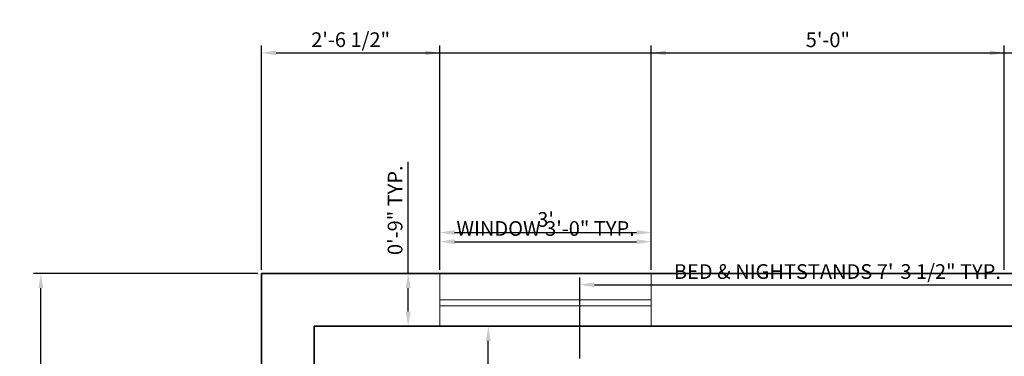
# Model space of a CAD drawing. Units: inches. Extents: x 2025 to 2528, y 1525 to 2336.
# Tile 13 of 18: x 2025 to 2192, y 2278 to 2336. Entities that reach past the tile are written whole.
import ezdxf

# ---------------------------------------------------------------- set-up
doc = ezdxf.new("R2010")
doc.units = ezdxf.units.IN
for name, color, linetype, lineweight in [('A-ANNO-DIMS', 2, 'Continuous', 18), ('A-GLAZ', 4, 'Continuous', 18), ('A-WALL', 7, 'Continuous', 35)]:
    doc.layers.add(name, color=color, linetype=linetype, lineweight=lineweight)
doc.styles.get("Standard").update_dxf_attribs({"font": 'arial.ttf'})
doc.dimstyles.new('Copy of ISO-25', dxfattribs={"dimtxt": 2.5, "dimasz": 2.5, "dimexe": 1.25, "dimexo": 0.625, "dimtad": 1, "dimdec": 1, "dimlunit": 4, "dimtxsty": 'Standard', "dimcen": 2.5, "dimadec": 0, "dimazin": 0, "dimtfac": 1, "dimtdec": 1, "dimtmove": 0, "dimatfit": 3, "dimfxl": 1, "dimarcsym": 0})

# ---------------------------------------------------------------- blocks, each defined once
blk = doc.blocks.new('*D6')
at = {"layer": 'A-ANNO-DIMS', "color": 0, "lineweight": -2, "transparency": 16777216}
for p, q in [((2075.01, 2282.79), (2075.01, 2237.93)), ((2255.01, 2282.79), (2255.01, 2237.93)), ((2077.51, 2239.18), (2252.51, 2239.18))]:
    blk.add_line(p, q, dxfattribs=at)
at = {"layer": 'A-ANNO-DIMS', "color": 0, "transparency": 16777216}
for points in [[(2077.51, 2239.59), (2077.51, 2238.76), (2075.01, 2239.18)], [(2252.51, 2239.59), (2252.51, 2238.76), (2255.01, 2239.18)]]:
    blk.add_solid(points, dxfattribs=at)
at = {"layer": 'Defpoints', "color": 0, "transparency": 16777216}
for p in [(2075.01, 2283.41), (2255.01, 2283.41), (2255.01, 2239.18)]:
    blk.add_point(p, dxfattribs=at)
at = {"layer": 'A-ANNO-DIMS', "color": 0, "transparency": 16777216, "insert": (2165.01, 2241.08), "char_height": 2.5, "attachment_point": 5}
blk.add_mtext("15'", dxfattribs=at)
blk = doc.blocks.new('*D7')
at = {"layer": 'A-ANNO-DIMS', "color": 0, "lineweight": -2, "transparency": 16777216}
for p, q in [((2075.64, 2283.41), (2105.88, 2283.41)), ((2104.63, 2117.91), (2104.63, 2280.91)), ((2075.64, 2115.41), (2105.88, 2115.41))]:
    blk.add_line(p, q, dxfattribs=at)
at = {"layer": 'A-ANNO-DIMS', "color": 0, "transparency": 16777216}
for points in [[(2104.22, 2280.91), (2105.05, 2280.91), (2104.63, 2283.41)], [(2104.22, 2117.91), (2105.05, 2117.91), (2104.63, 2115.41)]]:
    blk.add_solid(points, dxfattribs=at)
at = {"layer": 'Defpoints', "color": 0, "transparency": 16777216}
for p in [(2075.01, 2283.41), (2104.63, 2283.41), (2075.01, 2115.41)]:
    blk.add_point(p, dxfattribs=at)
at = {"layer": 'A-ANNO-DIMS', "color": 0, "transparency": 16777216, "insert": (2102.75, 2199.41), "char_height": 2.5, "attachment_point": 5, "rotation": 90}
blk.add_mtext("14'", dxfattribs=at)
blk = doc.blocks.new('*D22')
at = {"layer": 'A-ANNO-DIMS', "color": 0, "lineweight": -2, "transparency": 16777216}
for p, q in [((2096.39, 2293.04), (2096.39, 2300.62)), ((2132.39, 2293.04), (2132.39, 2300.62)), ((2098.89, 2299.37), (2129.89, 2299.37))]:
    blk.add_line(p, q, dxfattribs=at)
at = {"layer": 'A-ANNO-DIMS', "color": 0, "transparency": 16777216}
for points in [[(2098.89, 2299.78), (2098.89, 2298.95), (2096.39, 2299.37)], [(2129.89, 2299.78), (2129.89, 2298.95), (2132.39, 2299.37)]]:
    blk.add_solid(points, dxfattribs=at)
at = {"layer": 'Defpoints', "color": 0, "transparency": 16777216}
for p in [(2132.39, 2299.37), (2096.39, 2292.41), (2132.39, 2292.41)]:
    blk.add_point(p, dxfattribs=at)
at = {"layer": 'A-ANNO-DIMS', "color": 0, "transparency": 16777216, "insert": (2114.39, 2301.27), "char_height": 2.5, "attachment_point": 5}
blk.add_mtext("3'", dxfattribs=at)
blk = doc.blocks.new('WIN-36-EXT')
for p, q in [((0, 0), (0, 9)), ((0, 9), (36, 9)), ((36, 9), (36, 0)), ((0, 4.5), (36, 4.5)), ((0, 3.5), (36, 3.5))]:
    blk.add_line(p, q)
blk = doc.blocks.new('*D54')
at = {"layer": 'A-ANNO-DIMS', "color": 0, "lineweight": -2, "transparency": 16777216}
for p, q in [((2096.39, 2293.04), (2096.39, 2299.06)), ((2132.39, 2293.04), (2132.39, 2299.06)), ((2098.89, 2297.81), (2129.89, 2297.81))]:
    blk.add_line(p, q, dxfattribs=at)
at = {"layer": 'A-ANNO-DIMS', "color": 0, "transparency": 16777216}
for points in [[(2098.89, 2298.23), (2098.89, 2297.4), (2096.39, 2297.81)], [(2129.89, 2298.23), (2129.89, 2297.4), (2132.39, 2297.81)]]:
    blk.add_solid(points, dxfattribs=at)
at = {"layer": 'Defpoints', "color": 0, "transparency": 16777216}
for p in [(2132.39, 2297.81), (2096.39, 2292.41), (2132.39, 2292.41)]:
    blk.add_point(p, dxfattribs=at)
at = {"layer": 'A-ANNO-DIMS', "color": 0, "transparency": 16777216, "insert": (2114.39, 2299.73), "char_height": 2.5, "attachment_point": 5}
blk.add_mtext('WINDOW 3\'-0" TYP.', dxfattribs=at)
blk = doc.blocks.new('*D55')
at = {"layer": 'A-ANNO-DIMS', "color": 0, "lineweight": -2, "transparency": 16777216}
for p, q in [((2090.99, 2292.41), (2090.99, 2311.4)), ((2095.76, 2292.41), (2089.74, 2292.41)), ((2090.99, 2285.91), (2090.99, 2289.91)), ((2095.76, 2283.41), (2089.74, 2283.41))]:
    blk.add_line(p, q, dxfattribs=at)
at = {"layer": 'A-ANNO-DIMS', "color": 0, "transparency": 16777216}
for points in [[(2090.57, 2289.91), (2091.41, 2289.91), (2090.99, 2292.41)], [(2090.57, 2285.91), (2091.41, 2285.91), (2090.99, 2283.41)]]:
    blk.add_solid(points, dxfattribs=at)
at = {"layer": 'Defpoints', "color": 0, "transparency": 16777216}
for p in [(2090.99, 2292.41), (2096.39, 2292.41), (2096.39, 2283.41)]:
    blk.add_point(p, dxfattribs=at)
at = {"layer": 'A-ANNO-DIMS', "color": 0, "transparency": 16777216, "insert": (2089.09, 2303.16), "char_height": 2.5, "attachment_point": 5, "rotation": 90}
blk.add_mtext('0\'-9" TYP.', dxfattribs=at)
blk = doc.blocks.new('*D56')
at = {"layer": 'A-ANNO-DIMS', "color": 0, "lineweight": -2, "transparency": 16777216}
for p, q in [((2120.21, 2277.94), (2120.21, 2291.73)), ((2207.93, 2277.94), (2207.93, 2291.73)), ((2122.71, 2290.48), (2205.43, 2290.48))]:
    blk.add_line(p, q, dxfattribs=at)
at = {"layer": 'A-ANNO-DIMS', "color": 0, "transparency": 16777216}
for points in [[(2122.71, 2290.89), (2122.71, 2290.06), (2120.21, 2290.48)], [(2205.43, 2290.89), (2205.43, 2290.06), (2207.93, 2290.48)]]:
    blk.add_solid(points, dxfattribs=at)
at = {"layer": 'Defpoints', "color": 0, "transparency": 16777216}
for p in [(2207.93, 2290.48), (2120.21, 2277.32), (2207.93, 2277.32)]:
    blk.add_point(p, dxfattribs=at)
at = {"layer": 'A-ANNO-DIMS', "color": 0, "transparency": 16777216, "insert": (2164.07, 2292.4), "char_height": 2.5, "attachment_point": 5}
blk.add_mtext('BED & NIGHTSTANDS 7\'-3 1/2" TYP.', dxfattribs=at)
blk = doc.blocks.new('*D60')
at = {"layer": 'A-ANNO-DIMS', "color": 0, "lineweight": -2, "transparency": 16777216}
for p, q in [((2066.01, 2293.04), (2066.01, 2331.21)), ((2096.39, 2293.04), (2096.39, 2331.21)), ((2068.51, 2329.96), (2093.89, 2329.96))]:
    blk.add_line(p, q, dxfattribs=at)
at = {"layer": 'A-ANNO-DIMS', "color": 0, "transparency": 16777216}
for points in [[(2068.51, 2330.38), (2068.51, 2329.55), (2066.01, 2329.96)], [(2093.89, 2330.38), (2093.89, 2329.55), (2096.39, 2329.96)]]:
    blk.add_solid(points, dxfattribs=at)
at = {"layer": 'Defpoints', "color": 0, "transparency": 16777216}
for p in [(2096.39, 2329.96), (2066.01, 2292.41), (2096.39, 2292.41)]:
    blk.add_point(p, dxfattribs=at)
at = {"layer": 'A-ANNO-DIMS', "color": 0, "transparency": 16777216, "insert": (2081.2, 2331.88), "char_height": 2.5, "attachment_point": 5}
blk.add_mtext('2\'-6 1/2"', dxfattribs=at)
blk = doc.blocks.new('*D61')
at = {"layer": 'A-ANNO-DIMS', "color": 0, "lineweight": -2, "transparency": 16777216}
for p, q in [((2132.39, 2293.04), (2132.39, 2331.21)), ((2192.48, 2293.04), (2192.48, 2331.21)), ((2134.89, 2329.96), (2189.98, 2329.96))]:
    blk.add_line(p, q, dxfattribs=at)
at = {"layer": 'A-ANNO-DIMS', "color": 0, "transparency": 16777216}
for points in [[(2134.89, 2330.38), (2134.89, 2329.55), (2132.39, 2329.96)], [(2189.98, 2330.38), (2189.98, 2329.55), (2192.48, 2329.96)]]:
    blk.add_solid(points, dxfattribs=at)
at = {"layer": 'Defpoints', "color": 0, "transparency": 16777216}
for p in [(2192.48, 2329.96), (2132.39, 2292.41), (2192.48, 2292.41)]:
    blk.add_point(p, dxfattribs=at)
at = {"layer": 'A-ANNO-DIMS', "color": 0, "transparency": 16777216, "insert": (2162.44, 2331.86), "char_height": 2.5, "attachment_point": 5}
blk.add_mtext('5\'-0"', dxfattribs=at)
blk = doc.blocks.new('*D79')
at = {"layer": 'A-ANNO-DIMS', "color": 0, "lineweight": -2, "transparency": 16777216}
for p, q in [((2066.01, 2293.04), (2066.01, 2331.21)), ((2489.01, 2293.04), (2489.01, 2331.21)), ((2068.51, 2329.96), (2486.51, 2329.96))]:
    blk.add_line(p, q, dxfattribs=at)
at = {"layer": 'A-ANNO-DIMS', "color": 0, "transparency": 16777216}
for points in [[(2068.51, 2330.38), (2068.51, 2329.55), (2066.01, 2329.96)], [(2486.51, 2330.38), (2486.51, 2329.55), (2489.01, 2329.96)]]:
    blk.add_solid(points, dxfattribs=at)
at = {"layer": 'Defpoints', "color": 0, "transparency": 16777216}
for p in [(2489.01, 2329.96), (2066.01, 2292.41), (2489.01, 2292.41)]:
    blk.add_point(p, dxfattribs=at)
at = {"layer": 'A-ANNO-DIMS', "color": 0, "transparency": 16777216, "insert": (2277.51, 2331.86), "char_height": 2.5, "attachment_point": 5}
blk.add_mtext('35\'-3"', dxfattribs=at)
blk = doc.blocks.new('*D80')
at = {"layer": 'A-ANNO-DIMS', "color": 0, "lineweight": -2, "transparency": 16777216}
for p, q in [((2065.39, 2292.41), (2027.21, 2292.41)), ((2028.46, 1566.91), (2028.46, 2289.91)), ((2285.39, 1564.41), (2027.21, 1564.41))]:
    blk.add_line(p, q, dxfattribs=at)
at = {"layer": 'A-ANNO-DIMS', "color": 0, "transparency": 16777216}
for points in [[(2028.05, 2289.91), (2028.88, 2289.91), (2028.46, 2292.41)], [(2028.05, 1566.91), (2028.88, 1566.91), (2028.46, 1564.41)]]:
    blk.add_solid(points, dxfattribs=at)
at = {"layer": 'Defpoints', "color": 0, "transparency": 16777216}
for p in [(2028.46, 2292.41), (2066.01, 2292.41), (2286.01, 1564.41)]:
    blk.add_point(p, dxfattribs=at)
at = {"layer": 'A-ANNO-DIMS', "color": 0, "transparency": 16777216, "insert": (2026.56, 1928.41), "char_height": 2.5, "attachment_point": 5, "rotation": 90}
blk.add_mtext('60\'-8"', dxfattribs=at)

msp = doc.modelspace()

# ---------------------------------------------------------------- linework, layer by layer
at = {"layer": 'A-WALL'}
for p, q in [((2066.01, 2292.41), (2246.01, 2292.41)), ((2066.01, 2292.41), (2066.01, 2283.41)), ((2066.01, 2283.41), (2066.01, 2115.41)), ((2075.01, 2283.41), (2246.01, 2283.41)), ((2075.01, 2283.41), (2075.01, 2115.41)), ((2075.01, 2283.41), (2255.01, 2283.41)), ((2075.01, 2283.41), (2075.01, 2115.41)), ((2075.01, 2283.41), (2096.39, 2283.41))]:
    msp.add_line(p, q, dxfattribs=at)

# ---------------------------------------------------------------- block references
at = {"layer": 'A-GLAZ'}
msp.add_blockref('WIN-36-EXT', (2096.39, 2283.41), dxfattribs=at)

# ---------------------------------------------------------------- dimensions: what is measured, and where the dimension line sits
at = {"layer": 'A-ANNO-DIMS'}
for base, p1, p2, override, picture, middle in [((2096.39, 2329.96), (2066.01, 2292.41), (2096.39, 2292.41), {"dimdec": 1, "dimlfac": 1, "dimrnd": 0, "dimzin": 1, "dimdsep": 46, "dimlunit": 4, "dimfrac": 2}, '*D60', (2081.2, 2331.88)), ((2489.01, 2329.96), (2066.01, 2292.41), (2489.01, 2292.41), {"dimdec": 1, "dimlfac": 1, "dimrnd": 0, "dimzin": 1, "dimdsep": 46, "dimlunit": 4, "dimfrac": 2}, '*D79', (2277.51, 2331.86)), ((2192.48, 2329.96), (2132.39, 2292.41), (2192.48, 2292.41), {"dimdec": 1, "dimlfac": 1, "dimrnd": 0, "dimzin": 1, "dimdsep": 46, "dimlunit": 4, "dimfrac": 2}, '*D61', (2162.44, 2331.86)), ((2132.39, 2299.37), (2096.39, 2292.41), (2132.39, 2292.41), {"dimclrd": 0, "dimclre": 0, "dimclrt": 0}, '*D22', (2114.39, 2301.27)), ((2255.01, 2239.18), (2075.01, 2283.41), (2255.01, 2283.41), {"dimclrd": 0, "dimclre": 0, "dimclrt": 0}, '*D6', (2165.01, 2241.08))]:
    dim = msp.add_linear_dim(base=base, p1=p1, p2=p2, dimstyle='Copy of ISO-25', override=override, dxfattribs=at)
    dim.commit()
    dim.dimension.update_dxf_attribs({"geometry": picture, "text_midpoint": middle})
dim = msp.add_linear_dim(base=(2090.99, 2292.41), p1=(2096.39, 2283.41), p2=(2096.39, 2292.41), angle=90, text='<> TYP.', dimstyle='Copy of ISO-25', override={"dimdec": 1, "dimlfac": 1, "dimrnd": 0, "dimzin": 1, "dimdsep": 46, "dimlunit": 4, "dimfrac": 2}, dxfattribs=at)
dim.commit()
dim.dimension.update_dxf_attribs({"geometry": '*D55', "text_midpoint": (2089.09, 2303.16)})
for base, p1, p2, text, picture, middle in [((2132.39, 2297.81), (2096.39, 2292.41), (2132.39, 2292.41), 'WINDOW <> TYP.', '*D54', (2114.39, 2299.73)), ((2207.93, 2290.48), (2120.21, 2277.32), (2207.93, 2277.32), 'BED & NIGHTSTANDS <> TYP.', '*D56', (2164.07, 2292.4))]:
    dim = msp.add_linear_dim(base=base, p1=p1, p2=p2, text=text, dimstyle='Copy of ISO-25', override={"dimdec": 1, "dimlfac": 1, "dimrnd": 0, "dimzin": 1, "dimdsep": 46, "dimlunit": 4, "dimfrac": 2}, dxfattribs=at)
    dim.commit()
    dim.dimension.update_dxf_attribs({"geometry": picture, "text_midpoint": middle})
for base, p1, p2, override, picture, middle in [((2028.46, 2292.41), (2286.01, 1564.41), (2066.01, 2292.41), {"dimdec": 1, "dimlfac": 1, "dimrnd": 0, "dimzin": 1, "dimdsep": 46, "dimlunit": 4, "dimfrac": 2}, '*D80', (2026.56, 1928.41)), ((2104.63, 2283.41), (2075.01, 2115.41), (2075.01, 2283.41), {"dimclrd": 0, "dimclre": 0, "dimclrt": 0}, '*D7', (2102.75, 2199.41))]:
    dim = msp.add_linear_dim(base=base, p1=p1, p2=p2, angle=90, dimstyle='Copy of ISO-25', override=override, dxfattribs=at)
    dim.commit()
    dim.dimension.update_dxf_attribs({"geometry": picture, "text_midpoint": middle})

doc.saveas('drawing.dxf')
